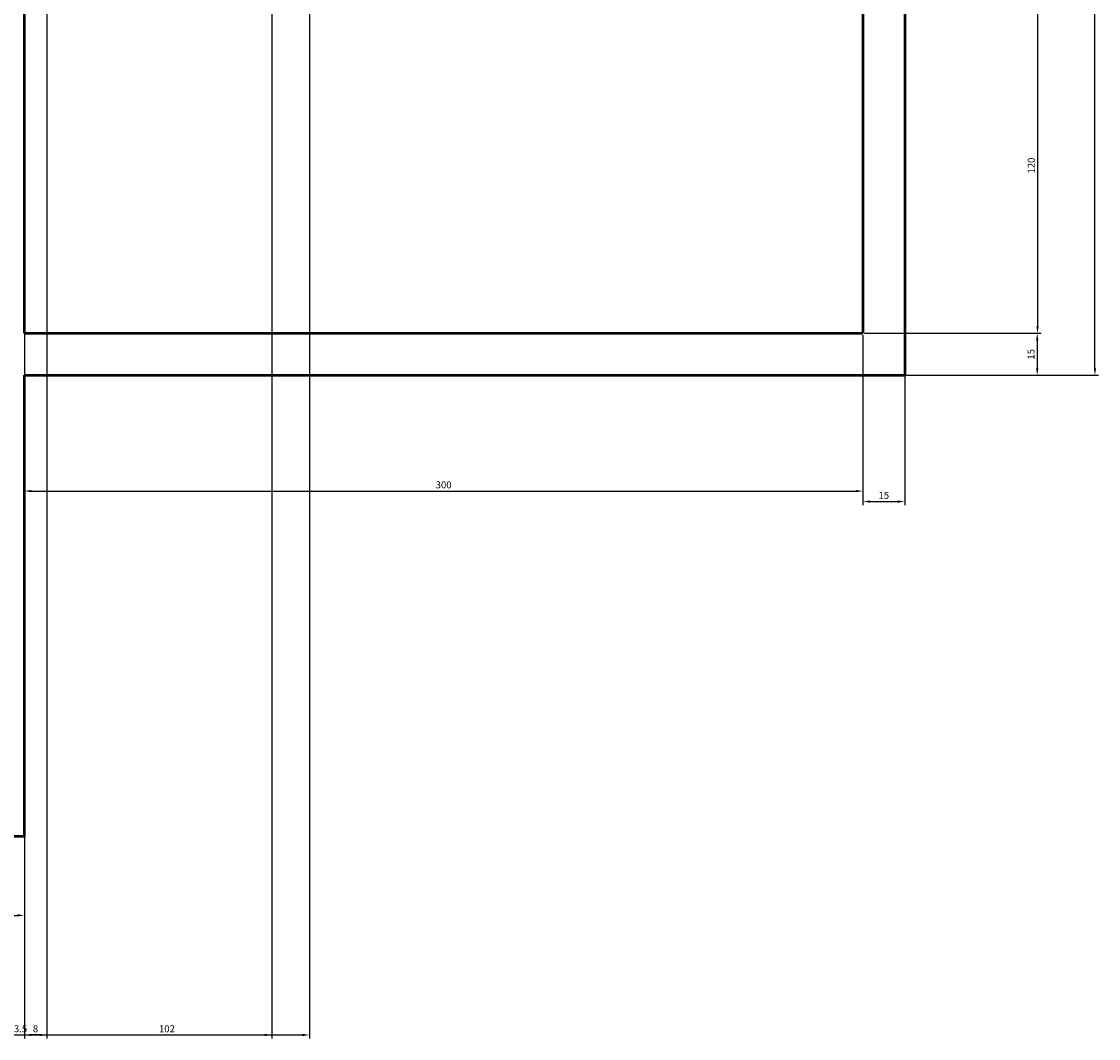
# Model space of a CAD drawing. Units: inches. Extents: x 604 to 3492, y -123 to 1737.
# Tile 6 of 20: x 1934 to 2319, y 216 to 579. Entities that reach past the tile are written whole.
import ezdxf

# ---------------------------------------------------------------- set-up
doc = ezdxf.new("R2010")
doc.units = ezdxf.units.IN
doc.layers.add('A-ANNO-DIMS', color=2, linetype='Continuous', lineweight=18)
doc.layers.add('A-WALL', color=7, linetype='Continuous', lineweight=50)
doc.styles.get("Standard").update_dxf_attribs({"font": 'arial.ttf'})
doc.dimstyles.new('ISO-25', dxfattribs={"dimtxt": 2.5, "dimasz": 2.5, "dimexe": 1.25, "dimexo": 0.625, "dimtad": 1, "dimtxsty": 'Standard', "dimcen": 2.5, "dimadec": 0, "dimazin": 0, "dimtfac": 1, "dimtmove": 0, "dimatfit": 3, "dimfxl": 1, "dimarcsym": 0})

# ---------------------------------------------------------------- blocks, each defined once
blk = doc.blocks.new('*D50')
at = {"layer": 'A-ANNO-DIMS', "color": 0, "lineweight": -2, "transparency": 16777216}
for p, q in [((2235.2, 587.7), (2298.31, 587.7)), ((2297.06, 585.2), (2297.06, 470.2)), ((2235.2, 467.7), (2298.31, 467.7))]:
    blk.add_line(p, q, dxfattribs=at)
at = {"layer": 'A-ANNO-DIMS', "color": 0, "transparency": 16777216}
for points in [[(2296.64, 585.2), (2297.48, 585.2), (2297.06, 587.7)], [(2296.64, 470.2), (2297.48, 470.2), (2297.06, 467.7)]]:
    blk.add_solid(points, dxfattribs=at)
at = {"layer": 'Defpoints', "color": 0, "transparency": 16777216}
for p in [(2234.57, 587.7), (2234.57, 467.7), (2297.06, 467.7)]:
    blk.add_point(p, dxfattribs=at)
at = {"layer": 'A-ANNO-DIMS', "color": 0, "transparency": 16777216, "insert": (2295.16, 527.7), "char_height": 2.5, "attachment_point": 5, "rotation": 90}
blk.add_mtext('120', dxfattribs=at)
blk = doc.blocks.new('*D51')
at = {"layer": 'A-ANNO-DIMS', "color": 0, "lineweight": -2, "transparency": 16777216}
for p, q in [((2235.2, 467.7), (2298.21, 467.7)), ((2296.96, 465.2), (2296.96, 455.2)), ((2235.2, 452.7), (2298.21, 452.7))]:
    blk.add_line(p, q, dxfattribs=at)
at = {"layer": 'A-ANNO-DIMS', "color": 0, "transparency": 16777216}
for points in [[(2296.54, 465.2), (2297.37, 465.2), (2296.96, 467.7)], [(2296.54, 455.2), (2297.37, 455.2), (2296.96, 452.7)]]:
    blk.add_solid(points, dxfattribs=at)
at = {"layer": 'Defpoints', "color": 0, "transparency": 16777216}
for p in [(2234.57, 467.7), (2234.57, 452.7), (2296.96, 452.7)]:
    blk.add_point(p, dxfattribs=at)
at = {"layer": 'A-ANNO-DIMS', "color": 0, "transparency": 16777216, "insert": (2295.06, 460.2), "char_height": 2.5, "attachment_point": 5, "rotation": 90}
blk.add_mtext('15', dxfattribs=at)
blk = doc.blocks.new('*D52')
at = {"layer": 'A-ANNO-DIMS', "color": 0, "lineweight": -2, "transparency": 16777216}
for p, q in [((2234.57, 467.08), (2234.57, 406.28)), ((2249.57, 467.08), (2249.57, 406.28)), ((2237.07, 407.53), (2247.07, 407.53))]:
    blk.add_line(p, q, dxfattribs=at)
at = {"layer": 'A-ANNO-DIMS', "color": 0, "transparency": 16777216}
for points in [[(2237.07, 407.94), (2237.07, 407.11), (2234.57, 407.53)], [(2247.07, 407.94), (2247.07, 407.11), (2249.57, 407.53)]]:
    blk.add_solid(points, dxfattribs=at)
at = {"layer": 'Defpoints', "color": 0, "transparency": 16777216}
for p in [(2234.57, 467.7), (2249.57, 467.7), (2249.57, 407.53)]:
    blk.add_point(p, dxfattribs=at)
at = {"layer": 'A-ANNO-DIMS', "color": 0, "transparency": 16777216, "insert": (2242.07, 409.43), "char_height": 2.5, "attachment_point": 5}
blk.add_mtext('15', dxfattribs=at)
blk = doc.blocks.new('*D53')
at = {"layer": 'A-ANNO-DIMS', "color": 0, "lineweight": -2, "transparency": 16777216}
for p, q in [((1934.57, 452.08), (1934.57, 410.03)), ((2234.57, 452.08), (2234.57, 410.03)), ((1937.07, 411.28), (2232.07, 411.28))]:
    blk.add_line(p, q, dxfattribs=at)
at = {"layer": 'A-ANNO-DIMS', "color": 0, "transparency": 16777216}
for points in [[(1937.07, 411.69), (1937.07, 410.86), (1934.57, 411.28)], [(2232.07, 411.69), (2232.07, 410.86), (2234.57, 411.28)]]:
    blk.add_solid(points, dxfattribs=at)
at = {"layer": 'Defpoints', "color": 0, "transparency": 16777216}
for p in [(1934.57, 452.7), (2234.57, 452.7), (2234.57, 411.28)]:
    blk.add_point(p, dxfattribs=at)
at = {"layer": 'A-ANNO-DIMS', "color": 0, "transparency": 16777216, "insert": (2084.57, 413.18), "char_height": 2.5, "attachment_point": 5}
blk.add_mtext('300', dxfattribs=at)
blk = doc.blocks.new('*D54')
at = {"layer": 'A-ANNO-DIMS', "color": 0, "lineweight": -2, "transparency": 16777216}
for p, q in [((1919.57, 302.08), (1919.57, 258.28)), ((1934.57, 302.08), (1934.57, 258.28)), ((1922.07, 259.53), (1932.07, 259.53))]:
    blk.add_line(p, q, dxfattribs=at)
at = {"layer": 'A-ANNO-DIMS', "color": 0, "transparency": 16777216}
for points in [[(1922.07, 259.95), (1922.07, 259.11), (1919.57, 259.53)], [(1932.07, 259.95), (1932.07, 259.11), (1934.57, 259.53)]]:
    blk.add_solid(points, dxfattribs=at)
at = {"layer": 'Defpoints', "color": 0, "transparency": 16777216}
for p in [(1919.57, 302.7), (1934.57, 302.7), (1934.57, 259.53)]:
    blk.add_point(p, dxfattribs=at)
at = {"layer": 'A-ANNO-DIMS', "color": 0, "transparency": 16777216, "insert": (1927.07, 261.43), "char_height": 2.5, "attachment_point": 5}
blk.add_mtext('15', dxfattribs=at)
blk = doc.blocks.new('*D70')
at = {"layer": 'A-ANNO-DIMS', "color": 0, "lineweight": -2, "transparency": 16777216}
for p, q in [((2250.2, 1287.7), (2318.86, 1287.7)), ((2317.61, 455.2), (2317.61, 1285.2)), ((2250.2, 452.7), (2318.86, 452.7))]:
    blk.add_line(p, q, dxfattribs=at)
at = {"layer": 'A-ANNO-DIMS', "color": 0, "transparency": 16777216}
for points in [[(2317.2, 1285.2), (2318.03, 1285.2), (2317.61, 1287.7)], [(2317.2, 455.2), (2318.03, 455.2), (2317.61, 452.7)]]:
    blk.add_solid(points, dxfattribs=at)
at = {"layer": 'Defpoints', "color": 0, "transparency": 16777216}
for p in [(2249.57, 1287.7), (2317.61, 1287.7), (2249.57, 452.7)]:
    blk.add_point(p, dxfattribs=at)
at = {"layer": 'A-ANNO-DIMS', "color": 0, "transparency": 16777216, "insert": (2315.71, 870.2), "char_height": 2.5, "attachment_point": 5, "rotation": 90}
blk.add_mtext('835', dxfattribs=at)
blk = doc.blocks.new('*D102')
at = {"layer": 'A-ANNO-DIMS', "color": 0, "lineweight": -2, "transparency": 16777216}
for p, q in [((1839.57, 972.08), (1839.57, 215.5)), ((2023.07, 972.08), (2023.07, 215.5)), ((1842.07, 216.75), (2020.57, 216.75))]:
    blk.add_line(p, q, dxfattribs=at)
at = {"layer": 'A-ANNO-DIMS', "color": 0, "transparency": 16777216}
for points in [[(1842.07, 217.17), (1842.07, 216.33), (1839.57, 216.75)], [(2020.57, 217.17), (2020.57, 216.33), (2023.07, 216.75)]]:
    blk.add_solid(points, dxfattribs=at)
at = {"layer": 'Defpoints', "color": 0, "transparency": 16777216}
for p in [(1839.57, 972.7), (2023.07, 972.7), (2023.07, 216.75)]:
    blk.add_point(p, dxfattribs=at)
at = {"layer": 'A-ANNO-DIMS', "color": 0, "transparency": 16777216, "insert": (1931.32, 218.65), "char_height": 2.5, "attachment_point": 5}
blk.add_mtext('183.5', dxfattribs=at)
blk = doc.blocks.new('*D104')
at = {"layer": 'A-ANNO-DIMS', "color": 0, "lineweight": -2, "transparency": 16777216}
for p, q in [((1934.57, 1272.08), (1934.57, 215.5)), ((2036.57, 1272.08), (2036.57, 215.5)), ((1937.07, 216.75), (2034.07, 216.75))]:
    blk.add_line(p, q, dxfattribs=at)
at = {"layer": 'A-ANNO-DIMS', "color": 0, "transparency": 16777216}
for points in [[(1937.07, 217.17), (1937.07, 216.33), (1934.57, 216.75)], [(2034.07, 217.17), (2034.07, 216.33), (2036.57, 216.75)]]:
    blk.add_solid(points, dxfattribs=at)
at = {"layer": 'Defpoints', "color": 0, "transparency": 16777216}
for p in [(1934.57, 1272.7), (2036.57, 1272.7), (2036.57, 216.75)]:
    blk.add_point(p, dxfattribs=at)
at = {"layer": 'A-ANNO-DIMS', "color": 0, "transparency": 16777216, "insert": (1985.57, 218.65), "char_height": 2.5, "attachment_point": 5}
blk.add_mtext('102', dxfattribs=at)
blk = doc.blocks.new('*D112')
at = {"layer": 'A-ANNO-DIMS', "color": 0, "lineweight": -2, "transparency": 16777216}
for p, q in [((1934.57, 972.08), (1934.57, 215.5)), ((1942.57, 962.08), (1942.57, 215.5)), ((1940.07, 216.75), (1937.07, 216.75))]:
    blk.add_line(p, q, dxfattribs=at)
at = {"layer": 'A-ANNO-DIMS', "color": 0, "transparency": 16777216}
for points in [[(1937.07, 217.17), (1937.07, 216.33), (1934.57, 216.75)], [(1940.07, 217.17), (1940.07, 216.33), (1942.57, 216.75)]]:
    blk.add_solid(points, dxfattribs=at)
at = {"layer": 'Defpoints', "color": 0, "transparency": 16777216}
for p in [(1934.57, 972.7), (1942.57, 962.7), (1934.57, 216.75)]:
    blk.add_point(p, dxfattribs=at)
at = {"layer": 'A-ANNO-DIMS', "color": 0, "transparency": 16777216, "insert": (1938.57, 218.65), "char_height": 2.5, "attachment_point": 5}
blk.add_mtext('8', dxfattribs=at)

msp = doc.modelspace()

# ---------------------------------------------------------------- linework, layer by layer
at = {"layer": 'A-WALL'}
for p, q in [((2249.5743, 1287.7004), (2249.5743, 452.7004)), ((1934.5743, 467.7004), (1934.5743, 587.7004)), ((2234.5743, 587.7004), (2234.5743, 467.7004)), ((1934.5743, 467.7004), (2234.5743, 467.7004)), ((1934.5743, 287.7004), (1934.5743, 452.7004)), ((1934.5743, 452.7004), (2234.5743, 452.7004)), ((2234.5743, 452.7004), (2249.5743, 452.7004)), ((1934.5743, 287.7004), (1574.5743, 287.7004))]:
    msp.add_line(p, q, dxfattribs=at)

# ---------------------------------------------------------------- dimensions: what is measured, and where the dimension line sits
at = {"layer": 'A-ANNO-DIMS'}
for p1, p2, distance, picture, middle in [((2249.5743, 452.7004), (2249.5743, 1287.7004), -68.0392, '*D70', (2315.7113, 870.2004)), ((2234.5743, 467.7004), (2249.5743, 467.7004), -60.1744, '*D52', (2242.0743, 409.4275))]:
    dim = msp.add_aligned_dim(p1=p1, p2=p2, distance=distance, dimstyle='ISO-25', override={"dimclrd": 0, "dimclre": 0, "dimclrt": 0}, dxfattribs=at)
    dim.commit()
    dim.dimension.update_dxf_attribs({"geometry": picture, "text_midpoint": middle})
for base, p1, p2, override, picture, middle in [((2036.5743, 216.7504), (1934.5743, 1272.7004), (2036.5743, 1272.7004), {"dimdec": 0, "dimlfac": 1, "dimrnd": 0, "dimzin": 0, "dimdsep": 46, "dimlunit": 2}, '*D104', (1985.5743, 218.6519)), ((2023.0743, 216.7504), (1839.5743, 972.7004), (2023.0743, 972.7004), {"dimdec": 1, "dimlfac": 1, "dimrnd": 0, "dimzin": 0, "dimdsep": 46, "dimlunit": 2}, '*D102', (1931.3243, 218.6527)), ((1934.5743, 216.7504), (1942.5743, 962.7004), (1934.5743, 972.7004), {"dimdec": 0, "dimlfac": 1, "dimrnd": 0, "dimzin": 0, "dimdsep": 46, "dimlunit": 2}, '*D112', (1938.5743, 218.6519)), ((2234.5743, 411.276), (1934.5743, 452.7004), (2234.5743, 452.7004), {"dimclrd": 0, "dimclre": 0, "dimclrt": 0}, '*D53', (2084.5743, 413.1783)), ((1934.5743, 259.5302), (1919.5743, 302.7004), (1934.5743, 302.7004), {"dimclrd": 0, "dimclre": 0, "dimclrt": 0}, '*D54', (1927.0743, 261.4316))]:
    dim = msp.add_linear_dim(base=base, p1=p1, p2=p2, dimstyle='ISO-25', override=override, dxfattribs=at)
    dim.commit()
    dim.dimension.update_dxf_attribs({"geometry": picture, "text_midpoint": middle})
for base, p1, p2, picture, middle in [((2297.0616, 467.7004), (2234.5743, 587.7004), (2234.5743, 467.7004), '*D50', (2295.1601, 527.7004)), ((2296.9576, 452.7004), (2234.5743, 467.7004), (2234.5743, 452.7004), '*D51', (2295.0562, 460.2004))]:
    dim = msp.add_linear_dim(base=base, p1=p1, p2=p2, angle=90, dimstyle='ISO-25', override={"dimclrd": 0, "dimclre": 0, "dimclrt": 0}, dxfattribs=at)
    dim.commit()
    dim.dimension.update_dxf_attribs({"geometry": picture, "text_midpoint": middle})

doc.saveas('drawing.dxf')
